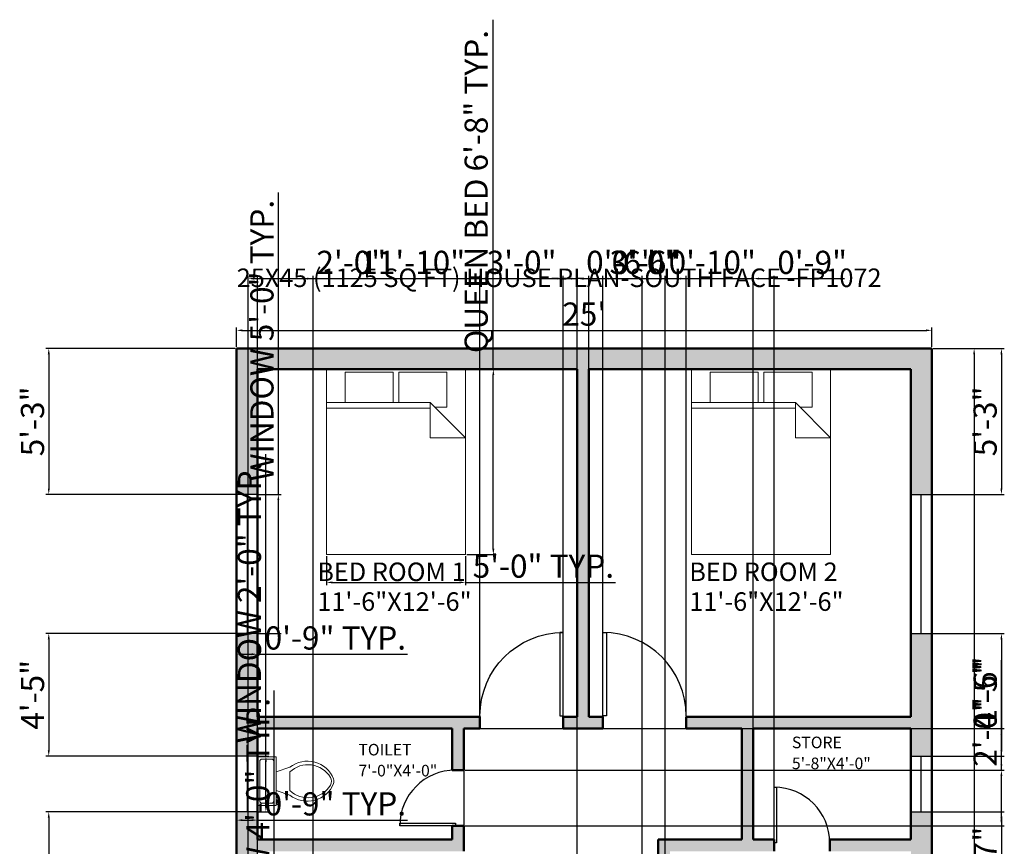
# Model space of a CAD drawing. Units: inches. Extents: x 3560 to 3985, y 1331 to 2044.
# Tile 2 of 2: x 3560 to 3985, y 1688 to 2044. Entities that reach past the tile are written whole.
import ezdxf

# ---------------------------------------------------------------- set-up
doc = ezdxf.new("R2010")
doc.units = ezdxf.units.IN
for name, color, linetype, lineweight in [('A-ANNO-DIMS', 5, 'Continuous', 18), ('A-ANNO-TEXT', 2, 'Continuous', 25), ('A-AREA-IDEN', 3, 'Continuous', 25), ('A-FLOR-FIXT', 9, 'Continuous', 18), ('A-FURN', 8, 'Continuous', 18), ('A-WALL-PATT', 7, 'Continuous', 13), ('DOOR', 6, 'Continuous', 25), ('WALL', 52, 'Continuous', 50), ('WINDOW', 4, 'Continuous', 25)]:
    doc.layers.add(name, color=color, linetype=linetype, lineweight=lineweight)
doc.styles.get("Standard").update_dxf_attribs({"font": 'arial.ttf'})
doc.dimstyles.new('ISO-25', dxfattribs={"dimtxt": 10, "dimasz": 2.5, "dimexe": 1.25, "dimexo": 0.625, "dimtad": 1, "dimdec": 1, "dimlunit": 3, "dimtxsty": 'Standard', "dimcen": 2.5, "dimadec": 0, "dimazin": 0, "dimtfac": 1, "dimtdec": 1, "dimtmove": 0, "dimatfit": 3, "dimfxl": 1, "dimarcsym": 0})

# ---------------------------------------------------------------- blocks, each defined once
blk = doc.blocks.new('*U5')
for p, q in [((0, 0), (0, -6)), ((40, 0), (40, -6))]:
    blk.add_line(p, q)
blk.add_lwpolyline([(0, 0), (0, 40), (1.75, 40), (1.75, 0)], close=True)
blk.add_arc((0, 0), 40, 0, 90)
blk = doc.blocks.new('*U7')
for p, q in [((9.5, -6), (9.5, -2)), ((-8, -8.5), (-8, -8)), ((-7, -8), (-7, -9.5)), ((-4, -8), (-6, -14)), ((4, -8), (6, -14)), ((-10, -8.5), (-8, -8.5)), ((-10, -9.5), (-10, -8.5)), ((-7, -9.5), (-10, -9.5)), ((4, -14), (-4, -14))]:
    blk.add_line(p, q)
blk.add_lwpolyline([(10.5, -8), (10.5, 0), (-10.5, 0), (-10.5, -8)], close=True)
for points in [[(-9.5, -2), (-9.5, -6)], [(8.5, -1), (-8.5, -1)], [(-8.5, -7), (8.5, -7)]]:
    blk.add_lwpolyline(points)
for centre, radius, start, end in [((-8.62, -1.88), 0.884, 81.8699, 188.1301), ((8.62, -1.88), 0.884, 351.8699, 98.1301), ((-8.62, -6.12), 0.884, 171.8699, 278.1301), ((8.62, -6.12), 0.884, 261.8699, 8.1301), ((3.52, -21.58), 12.17, 141.4691, 247.9714), ((4.2, -21.82), 11.33, 136.3677, 238.9468), ((-3.52, -21.58), 12.17, 292.0284, 38.5307), ((-4.2, -21.82), 11.33, 301.053, 43.6321), ((0, -27.88), 4, 245.7318, 294.2682), ((0, -29), 4, 254.8605, 285.1395)]:
    blk.add_arc(centre, radius, start, end)
blk = doc.blocks.new('Bed - Queen')
for p, q in [((0, -80.00003), (0, 0)), ((0, 0), (59.99999, 0)), ((59.99999, 0), (59.99999, -80.00003)), ((7.99999, -1.2), (28.79998, -1.2)), ((7.99999, -14.4), (7.99999, -1.2)), ((28.79998, -1.2), (28.79998, -14.4)), ((31.19999, -1.2), (51.99999, -1.2)), ((31.19999, -14.4), (31.19999, -1.2)), ((51.99999, -1.2), (51.99999, -16.4)), ((0, -14.4), (44.8, -14.4)), ((44.8, -16.8), (0, -16.8)), ((59.99999, -29.6), (44.8, -14.4)), ((44.8, -14.4), (44.8, -29.6)), ((51.99999, -16.4), (46.79936, -16.4)), ((44.8, -29.6), (59.99999, -29.6)), ((59.99999, -80.00003), (0, -80.00003))]:
    blk.add_line(p, q)
blk = doc.blocks.new('*D11')
at = {"layer": 'A-ANNO-DIMS', "color": 0, "lineweight": -2, "transparency": 16777216}
for p, q in [((3653.42, 1903.19), (3653.42, 1911.59)), ((3655.92, 1910.34), (3950.92, 1910.34)), ((3953.42, 1903.19), (3953.42, 1911.59))]:
    blk.add_line(p, q, dxfattribs=at)
at = {"layer": 'A-ANNO-DIMS', "color": 0, "transparency": 16777216}
for points in [[(3655.92, 1910.76), (3655.92, 1909.92), (3653.42, 1910.34)], [(3950.92, 1910.76), (3950.92, 1909.92), (3953.42, 1910.34)]]:
    blk.add_solid(points, dxfattribs=at)
at = {"layer": 'Defpoints', "color": 0, "transparency": 16777216}
for p in [(3953.42, 1910.34), (3653.42, 1902.56), (3953.42, 1902.56)]:
    blk.add_point(p, dxfattribs=at)
at = {"layer": 'A-ANNO-DIMS', "color": 0, "transparency": 16777216, "insert": (3803.42, 1916.07), "char_height": 10, "attachment_point": 5}
blk.add_mtext("25'", dxfattribs=at)
blk = doc.blocks.new('*D12')
at = {"layer": 'A-ANNO-DIMS', "color": 0, "lineweight": -2, "transparency": 16777216}
for p, q in [((3954.04, 1902.56), (3973, 1902.56)), ((3971.75, 1900.06), (3971.75, 1365.06)), ((3954.04, 1362.56), (3973, 1362.56))]:
    blk.add_line(p, q, dxfattribs=at)
at = {"layer": 'A-ANNO-DIMS', "color": 0, "transparency": 16777216}
for points in [[(3971.33, 1900.06), (3972.16, 1900.06), (3971.75, 1902.56)], [(3971.33, 1365.06), (3972.16, 1365.06), (3971.75, 1362.56)]]:
    blk.add_solid(points, dxfattribs=at)
at = {"layer": 'Defpoints', "color": 0, "transparency": 16777216}
for p in [(3953.42, 1902.56), (3953.42, 1362.56), (3971.75, 1362.56)]:
    blk.add_point(p, dxfattribs=at)
at = {"layer": 'A-ANNO-DIMS', "color": 0, "transparency": 16777216, "insert": (3966.04, 1633.18), "char_height": 10, "attachment_point": 5, "rotation": 90}
blk.add_mtext("45'", dxfattribs=at)
blk = doc.blocks.new('WIN-24IN')
for p, q in [((9, 24), (0, 24)), ((4.5, 24), (4.5, 0)), ((9, 0), (0, 0))]:
    blk.add_line(p, q)
blk = doc.blocks.new('WIN-60IN')
for p, q in [((9, 60), (0, 60)), ((4.5, 60), (4.5, 0)), ((9, 0), (0, 0))]:
    blk.add_line(p, q)
blk = doc.blocks.new('*D16')
at = {"layer": 'A-ANNO-DIMS', "color": 0, "lineweight": -2, "transparency": 16777216}
for p, q in [((3764.21, 1893.56), (3764.21, 2044.41)), ((3752.83, 1893.56), (3765.46, 1893.56)), ((3764.21, 1816.06), (3764.21, 1891.06)), ((3752.83, 1813.56), (3765.46, 1813.56))]:
    blk.add_line(p, q, dxfattribs=at)
at = {"layer": 'A-ANNO-DIMS', "color": 0, "transparency": 16777216}
for points in [[(3763.79, 1891.06), (3764.62, 1891.06), (3764.21, 1893.56)], [(3763.79, 1816.06), (3764.62, 1816.06), (3764.21, 1813.56)]]:
    blk.add_solid(points, dxfattribs=at)
at = {"layer": 'Defpoints', "color": 0, "transparency": 16777216}
for p in [(3752.21, 1893.56), (3764.21, 1893.56), (3752.21, 1813.56)]:
    blk.add_point(p, dxfattribs=at)
at = {"layer": 'A-ANNO-DIMS', "color": 0, "transparency": 16777216, "insert": (3758.1, 1970.24), "char_height": 10, "attachment_point": 5, "rotation": 90}
blk.add_mtext('QUEEN BED 6\'-8" TYP.', dxfattribs=at)
blk = doc.blocks.new('*D17')
at = {"layer": 'A-ANNO-DIMS', "color": 0, "lineweight": -2, "transparency": 16777216}
for p, q in [((3692.21, 1812.94), (3692.21, 1800.31)), ((3752.21, 1812.94), (3752.21, 1800.31)), ((3694.71, 1801.56), (3749.71, 1801.56)), ((3752.21, 1801.56), (3816.91, 1801.56))]:
    blk.add_line(p, q, dxfattribs=at)
at = {"layer": 'A-ANNO-DIMS', "color": 0, "transparency": 16777216}
for points in [[(3694.71, 1801.98), (3694.71, 1801.15), (3692.21, 1801.56)], [(3749.71, 1801.98), (3749.71, 1801.15), (3752.21, 1801.56)]]:
    blk.add_solid(points, dxfattribs=at)
at = {"layer": 'Defpoints', "color": 0, "transparency": 16777216}
for p in [(3692.21, 1813.56), (3752.21, 1813.56), (3752.21, 1801.56)]:
    blk.add_point(p, dxfattribs=at)
at = {"layer": 'A-ANNO-DIMS', "color": 0, "transparency": 16777216, "insert": (3785.81, 1807.29), "char_height": 10, "attachment_point": 5}
blk.add_mtext('5\'-0" TYP.', dxfattribs=at)
blk = doc.blocks.new('*D18')
at = {"layer": 'A-ANNO-DIMS', "color": 0, "lineweight": -2, "transparency": 16777216}
for p, q in [((3671.42, 1839.56), (3671.42, 1969.85)), ((3663.04, 1839.56), (3672.67, 1839.56)), ((3671.42, 1782.06), (3671.42, 1837.06)), ((3663.04, 1779.56), (3672.67, 1779.56))]:
    blk.add_line(p, q, dxfattribs=at)
at = {"layer": 'A-ANNO-DIMS', "color": 0, "transparency": 16777216}
for points in [[(3671, 1837.06), (3671.83, 1837.06), (3671.42, 1839.56)], [(3671, 1782.06), (3671.83, 1782.06), (3671.42, 1779.56)]]:
    blk.add_solid(points, dxfattribs=at)
at = {"layer": 'Defpoints', "color": 0, "transparency": 16777216}
for p in [(3662.42, 1839.56), (3671.42, 1839.56), (3662.42, 1779.56)]:
    blk.add_point(p, dxfattribs=at)
at = {"layer": 'A-ANNO-DIMS', "color": 0, "transparency": 16777216, "insert": (3665.62, 1905.96), "char_height": 10, "attachment_point": 5, "rotation": 90}
blk.add_mtext('WINDOW 5\'-0" TYP.', dxfattribs=at)
blk = doc.blocks.new('*D19')
at = {"layer": 'A-ANNO-DIMS', "color": 0, "lineweight": -2, "transparency": 16777216}
for p, q in [((3653.42, 1778.94), (3653.42, 1769.31)), ((3662.42, 1778.94), (3662.42, 1769.31)), ((3655.92, 1770.56), (3659.92, 1770.56)), ((3662.42, 1770.56), (3727.12, 1770.56))]:
    blk.add_line(p, q, dxfattribs=at)
at = {"layer": 'A-ANNO-DIMS', "color": 0, "transparency": 16777216}
for points in [[(3655.92, 1770.98), (3655.92, 1770.15), (3653.42, 1770.56)], [(3659.92, 1770.98), (3659.92, 1770.15), (3662.42, 1770.56)]]:
    blk.add_solid(points, dxfattribs=at)
at = {"layer": 'Defpoints', "color": 0, "transparency": 16777216}
for p in [(3653.42, 1779.56), (3662.42, 1779.56), (3662.42, 1770.56)]:
    blk.add_point(p, dxfattribs=at)
at = {"layer": 'A-ANNO-DIMS', "color": 0, "transparency": 16777216, "insert": (3696.02, 1776.29), "char_height": 10, "attachment_point": 5}
blk.add_mtext('0\'-9" TYP.', dxfattribs=at)
blk = doc.blocks.new('*D20')
at = {"layer": 'A-ANNO-DIMS', "color": 0, "lineweight": -2, "transparency": 16777216}
for p, q in [((3669.62, 1624.56), (3669.62, 1754.85)), ((3663.04, 1624.56), (3670.87, 1624.56)), ((3669.62, 1579.06), (3669.62, 1622.06)), ((3663.04, 1576.56), (3670.87, 1576.56))]:
    blk.add_line(p, q, dxfattribs=at)
at = {"layer": 'A-ANNO-DIMS', "color": 0, "transparency": 16777216}
for points in [[(3669.2, 1622.06), (3670.03, 1622.06), (3669.62, 1624.56)], [(3669.2, 1579.06), (3670.03, 1579.06), (3669.62, 1576.56)]]:
    blk.add_solid(points, dxfattribs=at)
at = {"layer": 'Defpoints', "color": 0, "transparency": 16777216}
for p in [(3662.42, 1624.56), (3669.62, 1624.56), (3662.42, 1576.56)]:
    blk.add_point(p, dxfattribs=at)
at = {"layer": 'A-ANNO-DIMS', "color": 0, "transparency": 16777216, "insert": (3663.82, 1690.96), "char_height": 10, "attachment_point": 5, "rotation": 90}
blk.add_mtext('WINDOW 4\'-0" TYP.', dxfattribs=at)
blk = doc.blocks.new('*D22')
at = {"layer": 'A-ANNO-DIMS', "color": 0, "lineweight": -2, "transparency": 16777216}
for p, q in [((3666.02, 1726.56), (3666.02, 1856.85)), ((3663.04, 1726.56), (3667.27, 1726.56)), ((3666.02, 1705.06), (3666.02, 1724.06)), ((3663.04, 1702.56), (3667.27, 1702.56))]:
    blk.add_line(p, q, dxfattribs=at)
at = {"layer": 'A-ANNO-DIMS', "color": 0, "transparency": 16777216}
for points in [[(3665.6, 1724.06), (3666.43, 1724.06), (3666.02, 1726.56)], [(3665.6, 1705.06), (3666.43, 1705.06), (3666.02, 1702.56)]]:
    blk.add_solid(points, dxfattribs=at)
at = {"layer": 'Defpoints', "color": 0, "transparency": 16777216}
for p in [(3662.42, 1726.56), (3666.02, 1726.56), (3662.42, 1702.56)]:
    blk.add_point(p, dxfattribs=at)
at = {"layer": 'A-ANNO-DIMS', "color": 0, "transparency": 16777216, "insert": (3660.22, 1792.96), "char_height": 10, "attachment_point": 5, "rotation": 90}
blk.add_mtext('WINDOW 2\'-0" TYP.', dxfattribs=at)
blk = doc.blocks.new('*D23')
at = {"layer": 'A-ANNO-DIMS', "color": 0, "lineweight": -2, "transparency": 16777216}
for p, q in [((3653.42, 1701.94), (3653.42, 1697.71)), ((3662.42, 1701.94), (3662.42, 1697.71)), ((3655.92, 1698.96), (3659.92, 1698.96)), ((3662.42, 1698.96), (3727.12, 1698.96))]:
    blk.add_line(p, q, dxfattribs=at)
at = {"layer": 'A-ANNO-DIMS', "color": 0, "transparency": 16777216}
for points in [[(3655.92, 1699.38), (3655.92, 1698.55), (3653.42, 1698.96)], [(3659.92, 1699.38), (3659.92, 1698.55), (3662.42, 1698.96)]]:
    blk.add_solid(points, dxfattribs=at)
at = {"layer": 'Defpoints', "color": 0, "transparency": 16777216}
for p in [(3653.42, 1702.56), (3662.42, 1702.56), (3662.42, 1698.96)]:
    blk.add_point(p, dxfattribs=at)
at = {"layer": 'A-ANNO-DIMS', "color": 0, "transparency": 16777216, "insert": (3696.02, 1704.69), "char_height": 10, "attachment_point": 5}
blk.add_mtext('0\'-9" TYP.', dxfattribs=at)
blk = doc.blocks.new('*D28')
at = {"layer": 'A-ANNO-DIMS', "color": 0, "lineweight": -2, "transparency": 16777216}
for p, q in [((3652.79, 1902.56), (3571.07, 1902.56)), ((3572.32, 1900.06), (3572.32, 1842.06)), ((3652.79, 1839.56), (3571.07, 1839.56))]:
    blk.add_line(p, q, dxfattribs=at)
at = {"layer": 'A-ANNO-DIMS', "color": 0, "transparency": 16777216}
for points in [[(3571.9, 1900.06), (3572.73, 1900.06), (3572.32, 1902.56)], [(3571.9, 1842.06), (3572.73, 1842.06), (3572.32, 1839.56)]]:
    blk.add_solid(points, dxfattribs=at)
at = {"layer": 'Defpoints', "color": 0, "transparency": 16777216}
for p in [(3653.42, 1902.56), (3572.32, 1839.56), (3653.42, 1839.56)]:
    blk.add_point(p, dxfattribs=at)
at = {"layer": 'A-ANNO-DIMS', "color": 0, "transparency": 16777216, "insert": (3566.58, 1871.06), "char_height": 10, "attachment_point": 5, "rotation": 90}
blk.add_mtext('5\'-3"', dxfattribs=at)
blk = doc.blocks.new('*D29')
at = {"layer": 'A-ANNO-DIMS', "color": 0, "lineweight": -2, "transparency": 16777216}
for p, q in [((3652.79, 1779.56), (3571.07, 1779.56)), ((3572.32, 1777.06), (3572.32, 1729.06)), ((3652.79, 1726.56), (3571.07, 1726.56))]:
    blk.add_line(p, q, dxfattribs=at)
at = {"layer": 'A-ANNO-DIMS', "color": 0, "transparency": 16777216}
for points in [[(3571.9, 1777.06), (3572.73, 1777.06), (3572.32, 1779.56)], [(3571.9, 1729.06), (3572.73, 1729.06), (3572.32, 1726.56)]]:
    blk.add_solid(points, dxfattribs=at)
at = {"layer": 'Defpoints', "color": 0, "transparency": 16777216}
for p in [(3653.42, 1779.56), (3572.32, 1726.56), (3653.42, 1726.56)]:
    blk.add_point(p, dxfattribs=at)
at = {"layer": 'A-ANNO-DIMS', "color": 0, "transparency": 16777216, "insert": (3566.61, 1753.06), "char_height": 10, "attachment_point": 5, "rotation": 90}
blk.add_mtext('4\'-5"', dxfattribs=at)
blk = doc.blocks.new('*D30')
at = {"layer": 'A-ANNO-DIMS', "color": 0, "lineweight": -2, "transparency": 16777216}
for p, q in [((3652.79, 1702.56), (3571.07, 1702.56)), ((3572.32, 1700.06), (3572.32, 1627.06)), ((3652.79, 1624.56), (3571.07, 1624.56))]:
    blk.add_line(p, q, dxfattribs=at)
at = {"layer": 'A-ANNO-DIMS', "color": 0, "transparency": 16777216}
for points in [[(3571.9, 1700.06), (3572.73, 1700.06), (3572.32, 1702.56)], [(3571.9, 1627.06), (3572.73, 1627.06), (3572.32, 1624.56)]]:
    blk.add_solid(points, dxfattribs=at)
at = {"layer": 'Defpoints', "color": 0, "transparency": 16777216}
for p in [(3653.42, 1702.56), (3572.32, 1624.56), (3653.42, 1624.56)]:
    blk.add_point(p, dxfattribs=at)
at = {"layer": 'A-ANNO-DIMS', "color": 0, "transparency": 16777216, "insert": (3566.59, 1663.56), "char_height": 10, "attachment_point": 5, "rotation": 90}
blk.add_mtext('6\'-6"', dxfattribs=at)
blk = doc.blocks.new('*D31')
at = {"layer": 'A-ANNO-DIMS', "color": 0, "lineweight": -2, "transparency": 16777216}
for p, q in [((3954.04, 1902.56), (3984.77, 1902.56)), ((3983.52, 1900.06), (3983.52, 1842.06)), ((3954.04, 1839.56), (3984.77, 1839.56))]:
    blk.add_line(p, q, dxfattribs=at)
at = {"layer": 'A-ANNO-DIMS', "color": 0, "transparency": 16777216}
for points in [[(3983.1, 1900.06), (3983.93, 1900.06), (3983.52, 1902.56)], [(3983.1, 1842.06), (3983.93, 1842.06), (3983.52, 1839.56)]]:
    blk.add_solid(points, dxfattribs=at)
at = {"layer": 'Defpoints', "color": 0, "transparency": 16777216}
for p in [(3953.42, 1902.56), (3953.42, 1839.56), (3983.52, 1839.56)]:
    blk.add_point(p, dxfattribs=at)
at = {"layer": 'A-ANNO-DIMS', "color": 0, "transparency": 16777216, "insert": (3977.78, 1871.06), "char_height": 10, "attachment_point": 5, "rotation": 90}
blk.add_mtext('5\'-3"', dxfattribs=at)
blk = doc.blocks.new('*D32')
at = {"layer": 'A-ANNO-DIMS', "color": 0, "lineweight": -2, "transparency": 16777216}
for p, q in [((3954.04, 1779.56), (3984.77, 1779.56)), ((3983.52, 1777.06), (3983.52, 1729.06)), ((3954.04, 1726.56), (3984.77, 1726.56))]:
    blk.add_line(p, q, dxfattribs=at)
at = {"layer": 'A-ANNO-DIMS', "color": 0, "transparency": 16777216}
for points in [[(3983.1, 1777.06), (3983.93, 1777.06), (3983.52, 1779.56)], [(3983.1, 1729.06), (3983.93, 1729.06), (3983.52, 1726.56)]]:
    blk.add_solid(points, dxfattribs=at)
at = {"layer": 'Defpoints', "color": 0, "transparency": 16777216}
for p in [(3953.42, 1779.56), (3953.42, 1726.56), (3983.52, 1726.56)]:
    blk.add_point(p, dxfattribs=at)
at = {"layer": 'A-ANNO-DIMS', "color": 0, "transparency": 16777216, "insert": (3977.81, 1753.06), "char_height": 10, "attachment_point": 5, "rotation": 90}
blk.add_mtext('4\'-5"', dxfattribs=at)
blk = doc.blocks.new('*D33')
at = {"layer": 'A-ANNO-DIMS', "color": 0, "lineweight": -2, "transparency": 16777216}
for p, q in [((3954.04, 1702.56), (3984.77, 1702.56)), ((3983.52, 1700.06), (3983.52, 1662.06)), ((3954.04, 1659.56), (3984.77, 1659.56))]:
    blk.add_line(p, q, dxfattribs=at)
at = {"layer": 'A-ANNO-DIMS', "color": 0, "transparency": 16777216}
for points in [[(3983.1, 1700.06), (3983.93, 1700.06), (3983.52, 1702.56)], [(3983.1, 1662.06), (3983.93, 1662.06), (3983.52, 1659.56)]]:
    blk.add_solid(points, dxfattribs=at)
at = {"layer": 'Defpoints', "color": 0, "transparency": 16777216}
for p in [(3953.42, 1702.56), (3953.42, 1659.56), (3983.52, 1659.56)]:
    blk.add_point(p, dxfattribs=at)
at = {"layer": 'A-ANNO-DIMS', "color": 0, "transparency": 16777216, "insert": (3977.78, 1681.06), "char_height": 10, "attachment_point": 5, "rotation": 90}
blk.add_mtext('3\'-7"', dxfattribs=at)
blk = doc.blocks.new('*D36')
at = {"layer": 'A-ANNO-DIMS', "color": 0, "lineweight": -2, "transparency": 16777216}
for p, q in [((3662.42, 1517.19), (3662.42, 1933.91)), ((3686.42, 1517.19), (3686.42, 1933.91)), ((3664.92, 1932.66), (3683.92, 1932.66)), ((3686.42, 1932.66), (3716.92, 1932.66))]:
    blk.add_line(p, q, dxfattribs=at)
at = {"layer": 'A-ANNO-DIMS', "color": 0, "transparency": 16777216}
for points in [[(3664.92, 1933.08), (3664.92, 1932.25), (3662.42, 1932.66)], [(3683.92, 1933.08), (3683.92, 1932.25), (3686.42, 1932.66)]]:
    blk.add_solid(points, dxfattribs=at)
at = {"layer": 'Defpoints', "color": 0, "transparency": 16777216}
for p in [(3686.42, 1932.66), (3662.42, 1516.56), (3686.42, 1516.56)]:
    blk.add_point(p, dxfattribs=at)
at = {"layer": 'A-ANNO-DIMS', "color": 0, "transparency": 16777216, "insert": (3702.92, 1938.39), "char_height": 10, "attachment_point": 5}
blk.add_mtext('2\'-0"', dxfattribs=at)
blk = doc.blocks.new('*D40')
at = {"layer": 'A-ANNO-DIMS', "color": 0, "lineweight": -2, "transparency": 16777216}
for p, q in [((3758.42, 1744.19), (3758.42, 1933.91)), ((3794.42, 1744.19), (3794.42, 1933.91)), ((3760.92, 1932.66), (3791.92, 1932.66))]:
    blk.add_line(p, q, dxfattribs=at)
at = {"layer": 'A-ANNO-DIMS', "color": 0, "transparency": 16777216}
for points in [[(3760.92, 1933.08), (3760.92, 1932.25), (3758.42, 1932.66)], [(3791.92, 1933.08), (3791.92, 1932.25), (3794.42, 1932.66)]]:
    blk.add_solid(points, dxfattribs=at)
at = {"layer": 'Defpoints', "color": 0, "transparency": 16777216}
for p in [(3794.42, 1932.66), (3758.42, 1743.56), (3794.42, 1743.56)]:
    blk.add_point(p, dxfattribs=at)
at = {"layer": 'A-ANNO-DIMS', "color": 0, "transparency": 16777216, "insert": (3776.42, 1938.4), "char_height": 10, "attachment_point": 5}
blk.add_mtext('3\'-0"', dxfattribs=at)
blk = doc.blocks.new('*D41')
at = {"layer": 'A-ANNO-DIMS', "color": 0, "lineweight": -2, "transparency": 16777216}
for p, q in [((3794.42, 1744.19), (3794.42, 1933.91)), ((3800.42, 1744.19), (3800.42, 1933.91)), ((3791.92, 1932.66), (3789.42, 1932.66)), ((3794.42, 1932.66), (3800.42, 1932.66)), ((3802.92, 1932.66), (3833.25, 1932.66))]:
    blk.add_line(p, q, dxfattribs=at)
at = {"layer": 'A-ANNO-DIMS', "color": 0, "transparency": 16777216}
for points in [[(3791.92, 1933.08), (3791.92, 1932.25), (3794.42, 1932.66)], [(3802.92, 1933.08), (3802.92, 1932.25), (3800.42, 1932.66)]]:
    blk.add_solid(points, dxfattribs=at)
at = {"layer": 'Defpoints', "color": 0, "transparency": 16777216}
for p in [(3800.42, 1932.66), (3794.42, 1743.56), (3800.42, 1743.56)]:
    blk.add_point(p, dxfattribs=at)
at = {"layer": 'A-ANNO-DIMS', "color": 0, "transparency": 16777216, "insert": (3819.33, 1938.39), "char_height": 10, "attachment_point": 5}
blk.add_mtext('0\'-6"', dxfattribs=at)
blk = doc.blocks.new('*D42')
at = {"layer": 'A-ANNO-DIMS', "color": 0, "lineweight": -2, "transparency": 16777216}
for p, q in [((3805.42, 1744.19), (3805.42, 1933.91)), ((3811.42, 1744.19), (3811.42, 1933.91)), ((3802.92, 1932.66), (3800.42, 1932.66)), ((3805.42, 1932.66), (3811.42, 1932.66)), ((3813.92, 1932.66), (3844.25, 1932.66))]:
    blk.add_line(p, q, dxfattribs=at)
at = {"layer": 'A-ANNO-DIMS', "color": 0, "transparency": 16777216}
for points in [[(3802.92, 1933.08), (3802.92, 1932.25), (3805.42, 1932.66)], [(3813.92, 1933.08), (3813.92, 1932.25), (3811.42, 1932.66)]]:
    blk.add_solid(points, dxfattribs=at)
at = {"layer": 'Defpoints', "color": 0, "transparency": 16777216}
for p in [(3811.42, 1932.66), (3805.42, 1743.56), (3811.42, 1743.56)]:
    blk.add_point(p, dxfattribs=at)
at = {"layer": 'A-ANNO-DIMS', "color": 0, "transparency": 16777216, "insert": (3830.33, 1938.39), "char_height": 10, "attachment_point": 5}
blk.add_mtext('0\'-6"', dxfattribs=at)
blk = doc.blocks.new('*D43')
at = {"layer": 'A-ANNO-DIMS', "color": 0, "lineweight": -2, "transparency": 16777216}
for p, q in [((3811.42, 1744.19), (3811.42, 1933.91)), ((3847.42, 1744.19), (3847.42, 1933.91)), ((3813.92, 1932.66), (3844.92, 1932.66))]:
    blk.add_line(p, q, dxfattribs=at)
at = {"layer": 'A-ANNO-DIMS', "color": 0, "transparency": 16777216}
for points in [[(3813.92, 1933.08), (3813.92, 1932.25), (3811.42, 1932.66)], [(3844.92, 1933.08), (3844.92, 1932.25), (3847.42, 1932.66)]]:
    blk.add_solid(points, dxfattribs=at)
at = {"layer": 'Defpoints', "color": 0, "transparency": 16777216}
for p in [(3847.42, 1932.66), (3811.42, 1743.56), (3847.42, 1743.56)]:
    blk.add_point(p, dxfattribs=at)
at = {"layer": 'A-ANNO-DIMS', "color": 0, "transparency": 16777216, "insert": (3829.42, 1938.4), "char_height": 10, "attachment_point": 5}
blk.add_mtext('3\'-0"', dxfattribs=at)
blk = doc.blocks.new('*D45')
at = {"layer": 'A-ANNO-DIMS', "color": 0, "lineweight": -2, "transparency": 16777216}
for p, q in [((3876.42, 1691.19), (3876.42, 1933.91)), ((3885.42, 1691.19), (3885.42, 1933.91)), ((3878.92, 1932.66), (3882.92, 1932.66)), ((3885.42, 1932.66), (3915.75, 1932.66))]:
    blk.add_line(p, q, dxfattribs=at)
at = {"layer": 'A-ANNO-DIMS', "color": 0, "transparency": 16777216}
for points in [[(3878.92, 1933.08), (3878.92, 1932.25), (3876.42, 1932.66)], [(3882.92, 1933.08), (3882.92, 1932.25), (3885.42, 1932.66)]]:
    blk.add_solid(points, dxfattribs=at)
at = {"layer": 'Defpoints', "color": 0, "transparency": 16777216}
for p in [(3885.42, 1932.66), (3876.42, 1690.56), (3885.42, 1690.56)]:
    blk.add_point(p, dxfattribs=at)
at = {"layer": 'A-ANNO-DIMS', "color": 0, "transparency": 16777216, "insert": (3901.83, 1938.39), "char_height": 10, "attachment_point": 5}
blk.add_mtext('0\'-9"', dxfattribs=at)
blk = doc.blocks.new('*D47')
at = {"layer": 'A-ANNO-DIMS', "color": 0, "lineweight": -2, "transparency": 16777216}
for p, q in [((3983.52, 1720.56), (3983.52, 1751.07)), ((3752.04, 1720.56), (3984.77, 1720.56)), ((3983.52, 1699.06), (3983.52, 1718.06)), ((3752.04, 1696.56), (3984.77, 1696.56))]:
    blk.add_line(p, q, dxfattribs=at)
at = {"layer": 'A-ANNO-DIMS', "color": 0, "transparency": 16777216}
for points in [[(3983.1, 1718.06), (3983.93, 1718.06), (3983.52, 1720.56)], [(3983.1, 1699.06), (3983.93, 1699.06), (3983.52, 1696.56)]]:
    blk.add_solid(points, dxfattribs=at)
at = {"layer": 'Defpoints', "color": 0, "transparency": 16777216}
for p in [(3751.42, 1720.56), (3983.52, 1720.56), (3751.42, 1696.56)]:
    blk.add_point(p, dxfattribs=at)
at = {"layer": 'A-ANNO-DIMS', "color": 0, "transparency": 16777216, "insert": (3977.79, 1737.06), "char_height": 10, "attachment_point": 5, "rotation": 90}
blk.add_mtext('2\'-0"', dxfattribs=at)
blk = doc.blocks.new('*D48')
at = {"layer": 'A-ANNO-DIMS', "color": 0, "lineweight": -2, "transparency": 16777216}
for p, q in [((3983.52, 1738.56), (3983.52, 1767.95)), ((3752.04, 1738.56), (3984.77, 1738.56)), ((3983.52, 1723.06), (3983.52, 1736.06)), ((3752.04, 1720.56), (3984.77, 1720.56))]:
    blk.add_line(p, q, dxfattribs=at)
at = {"layer": 'A-ANNO-DIMS', "color": 0, "transparency": 16777216}
for points in [[(3983.1, 1736.06), (3983.93, 1736.06), (3983.52, 1738.56)], [(3983.1, 1723.06), (3983.93, 1723.06), (3983.52, 1720.56)]]:
    blk.add_solid(points, dxfattribs=at)
at = {"layer": 'Defpoints', "color": 0, "transparency": 16777216}
for p in [(3751.42, 1738.56), (3983.52, 1738.56), (3751.42, 1720.56)]:
    blk.add_point(p, dxfattribs=at)
at = {"layer": 'A-ANNO-DIMS', "color": 0, "transparency": 16777216, "insert": (3977.79, 1754.51), "char_height": 10, "attachment_point": 5, "rotation": 90}
blk.add_mtext('1\'-6"', dxfattribs=at)
blk = doc.blocks.new('*D52')
at = {"layer": 'A-ANNO-DIMS', "color": 0, "lineweight": -2, "transparency": 16777216}
for p, q in [((3658.42, 1372.19), (3658.42, 1933.91)), ((3800.42, 1372.19), (3800.42, 1933.91)), ((3660.92, 1932.66), (3797.92, 1932.66))]:
    blk.add_line(p, q, dxfattribs=at)
at = {"layer": 'A-ANNO-DIMS', "color": 0, "transparency": 16777216}
for points in [[(3660.92, 1933.08), (3660.92, 1932.25), (3658.42, 1932.66)], [(3797.92, 1933.08), (3797.92, 1932.25), (3800.42, 1932.66)]]:
    blk.add_solid(points, dxfattribs=at)
at = {"layer": 'Defpoints', "color": 0, "transparency": 16777216}
for p in [(3800.42, 1932.66), (3658.42, 1371.56), (3800.42, 1371.56)]:
    blk.add_point(p, dxfattribs=at)
at = {"layer": 'A-ANNO-DIMS', "color": 0, "transparency": 16777216, "insert": (3729.42, 1938.39), "char_height": 10, "attachment_point": 5}
blk.add_mtext('11\'-10"', dxfattribs=at)
blk = doc.blocks.new('*D53')
at = {"layer": 'A-ANNO-DIMS', "color": 0, "lineweight": -2, "transparency": 16777216}
for p, q in [((3828.42, 1372.19), (3828.42, 1933.91)), ((3838.42, 1372.19), (3838.42, 1933.91)), ((3830.92, 1932.66), (3835.92, 1932.66)), ((3838.42, 1932.66), (3876.52, 1932.66))]:
    blk.add_line(p, q, dxfattribs=at)
at = {"layer": 'A-ANNO-DIMS', "color": 0, "transparency": 16777216}
for points in [[(3830.92, 1933.08), (3830.92, 1932.25), (3828.42, 1932.66)], [(3835.92, 1933.08), (3835.92, 1932.25), (3838.42, 1932.66)]]:
    blk.add_solid(points, dxfattribs=at)
at = {"layer": 'Defpoints', "color": 0, "transparency": 16777216}
for p in [(3838.42, 1932.66), (3828.42, 1371.56), (3838.42, 1371.56)]:
    blk.add_point(p, dxfattribs=at)
at = {"layer": 'A-ANNO-DIMS', "color": 0, "transparency": 16777216, "insert": (3858.72, 1938.39), "char_height": 10, "attachment_point": 5}
blk.add_mtext('0\'-10"', dxfattribs=at)

msp = doc.modelspace()

# ---------------------------------------------------------------- hatches: boundary and pattern name
at = {"layer": 'A-WALL-PATT'}
h = msp.add_hatch(color=256, dxfattribs=at)
h.dxf.hatch_style = 1
h.paths.add_polyline_path([(3953.42, 1902.56), (3653.42, 1902.56), (3653.42, 1839.56), (3662.42, 1839.56), (3662.42, 1893.56), (3800.42, 1893.56), (3800.42, 1743.56), (3794.42, 1743.56), (3794.42, 1738.56), (3800.42, 1738.56), (3811.42, 1738.56), (3811.42, 1743.56), (3805.42, 1743.56), (3805.42, 1893.56), (3944.42, 1893.56), (3944.42, 1839.56), (3953.42, 1839.56)])
h = msp.add_hatch(color=256, dxfattribs=at)
h.dxf.hatch_style = 1
h.paths.add_polyline_path([(3758.42, 1743.56), (3662.42, 1743.56), (3662.42, 1779.56), (3653.42, 1779.56), (3653.42, 1726.56), (3662.42, 1726.56), (3662.42, 1738.56), (3746.42, 1738.56), (3746.42, 1720.56), (3751.42, 1720.56), (3751.42, 1738.56), (3758.42, 1738.56)])
h = msp.add_hatch(color=256, dxfattribs=at)
h.dxf.hatch_style = 1
h.paths.add_polyline_path([(3953.42, 1779.56), (3944.42, 1779.56), (3944.42, 1743.56), (3847.42, 1743.56), (3847.42, 1738.56), (3871.42, 1738.56), (3871.42, 1690.56), (3835.42, 1690.56), (3835.42, 1679.56), (3840.42, 1679.56), (3840.42, 1685.56), (3885.42, 1685.56), (3885.42, 1689.16), (3885.42, 1690.56), (3876.42, 1690.56), (3876.42, 1738.56), (3944.42, 1738.56), (3944.42, 1726.56), (3953.42, 1726.56)])
h = msp.add_hatch(color=256, dxfattribs=at)
h.dxf.hatch_style = 1
h.paths.add_polyline_path([(3662.42, 1685.56), (3751.42, 1685.56), (3751.42, 1696.56), (3747.82, 1696.56), (3746.42, 1696.56), (3746.42, 1690.56), (3662.42, 1690.56), (3662.42, 1702.56), (3653.42, 1702.56), (3653.42, 1624.56), (3662.42, 1624.56)])
h = msp.add_hatch(color=256, dxfattribs=at)
h.dxf.hatch_style = 1
h.paths.add_polyline_path([(3953.42, 1702.56), (3944.42, 1702.56), (3944.42, 1690.56), (3909.42, 1690.56), (3909.42, 1685.56), (3944.42, 1685.56), (3944.42, 1659.56), (3953.42, 1659.56)])

# ---------------------------------------------------------------- linework, layer by layer
at = {"layer": 'DOOR'}
for p, q in [((3758.42, 1738.56), (3794.42, 1738.56)), ((3811.42, 1738.56), (3847.42, 1738.56)), ((3751.42, 1720.56), (3751.42, 1696.56))]:
    msp.add_line(p, q, dxfattribs=at)
at = {"layer": 'WALL'}
for p, q in [((3653.42, 1902.56), (3953.42, 1902.56)), ((3653.42, 1902.56), (3653.42, 1362.56)), ((3953.42, 1902.56), (3953.42, 1362.56)), ((3662.42, 1893.56), (3800.42, 1893.56)), ((3662.42, 1893.56), (3662.42, 1743.56)), ((3800.42, 1893.56), (3800.42, 1743.56)), ((3805.42, 1893.56), (3805.42, 1743.56)), ((3805.42, 1893.56), (3944.42, 1893.56)), ((3944.42, 1893.56), (3944.42, 1743.56)), ((3662.42, 1743.56), (3758.42, 1743.56)), ((3758.42, 1743.56), (3758.42, 1738.56)), ((3794.42, 1743.56), (3794.42, 1738.56)), ((3794.42, 1743.56), (3800.42, 1743.56)), ((3805.42, 1743.56), (3811.42, 1743.56)), ((3811.42, 1743.56), (3811.42, 1738.56)), ((3847.42, 1743.56), (3847.42, 1738.56)), ((3847.42, 1743.56), (3944.42, 1743.56)), ((3662.42, 1738.56), (3746.42, 1738.56)), ((3662.42, 1738.56), (3662.42, 1690.56)), ((3746.42, 1738.56), (3746.42, 1720.56)), ((3751.42, 1738.56), (3751.42, 1720.56)), ((3751.42, 1738.56), (3758.42, 1738.56)), ((3794.42, 1738.56), (3800.42, 1738.56)), ((3800.42, 1738.56), (3811.42, 1738.56)), ((3847.42, 1738.56), (3871.42, 1738.56)), ((3871.42, 1738.56), (3871.42, 1690.56)), ((3876.42, 1738.56), (3876.42, 1690.56)), ((3876.42, 1738.56), (3944.42, 1738.56)), ((3944.42, 1738.56), (3944.42, 1690.56)), ((3746.42, 1720.56), (3751.42, 1720.56)), ((3746.42, 1696.56), (3751.42, 1696.56)), ((3746.42, 1696.56), (3746.42, 1690.56)), ((3751.42, 1696.56), (3751.42, 1685.56)), ((3662.42, 1690.56), (3746.42, 1690.56)), ((3835.42, 1690.56), (3871.42, 1690.56)), ((3835.42, 1690.56), (3835.42, 1679.56)), ((3876.42, 1690.56), (3885.42, 1690.56)), ((3885.42, 1690.56), (3885.42, 1685.56)), ((3909.42, 1690.56), (3909.42, 1685.56)), ((3909.42, 1690.56), (3944.42, 1690.56))]:
    msp.add_line(p, q, dxfattribs=at)

# ---------------------------------------------------------------- block references
at = {"layer": 'A-FLOR-FIXT', "rotation": 90}
msp.add_blockref('*U7', (3662.42, 1715.76), dxfattribs=at)
at = {"layer": 'A-FURN'}
for p in [(3692.21, 1893.56), (3849.77, 1893.56)]:
    msp.add_blockref('Bed - Queen', p, dxfattribs=at)
at = {"layer": 'DOOR'}
for p, xscale, yscale, zscale in [((3794.42, 1743.96), -0.8999999999999898, 0.8999999999999898, 0.8999999999999898), ((3811.42, 1743.96), 0.8999999999999898, 0.8999999999999898, 0.8999999999999898), ((3885.42, 1689.16), 0.5999999999999819, 0.5999999999999819, 0.5999999999999819)]:
    msp.add_blockref('*U5', p, dxfattribs=dict(at, xscale=xscale, yscale=yscale, zscale=zscale))
at = {"layer": 'DOOR', "xscale": 0.5999999999999782, "yscale": 0.5999999999999782, "zscale": 0.5999999999999782, "rotation": 89.99999999999902}
msp.add_blockref('*U5', (3747.82, 1696.56), dxfattribs=at)
at = {"layer": 'WINDOW'}
for name, p in [('WIN-60IN', (3653.42, 1779.56)), ('WIN-24IN', (3653.42, 1702.56))]:
    msp.add_blockref(name, p, dxfattribs=at)
at = {"layer": 'WINDOW', "rotation": 180}
for name, p in [('WIN-60IN', (3953.42, 1839.56)), ('WIN-24IN', (3953.42, 1726.56))]:
    msp.add_blockref(name, p, dxfattribs=at)

# ---------------------------------------------------------------- texts
at = {"layer": 'A-ANNO-TEXT'}
msp.add_text('25X45 (1125 SQ FT) HOUSE PLAN-SOUTH FACE -FP1072', height=8, dxfattribs=at).set_placement((3653.45, 1929.03))
at = {"layer": 'A-AREA-IDEN'}
for s, height, p in [('BED ROOM 1', 8, (3688.23, 1802.14)), ('BED ROOM 2', 8, (3848.79, 1802.14)), ('11\'-6"X12\'-6"', 8, (3688.23, 1789.29)), ('11\'-6"X12\'-6"', 8, (3848.79, 1789.29)), ('STORE', 5, (3893.09, 1730)), ('TOILET', 5, (3705.97, 1726.88)), ('5\'-8"X4\'-0"', 5, (3893.09, 1720.96)), ('7\'-0"X4\'-0"', 5, (3705.97, 1717.84))]:
    msp.add_text(s, height=height, dxfattribs=at).set_placement(p)

# ---------------------------------------------------------------- dimensions: what is measured, and where the dimension line sits
at = {"layer": 'A-ANNO-DIMS'}
for base, p1, p2, text, picture, middle in [((3764.21, 1893.56), (3752.21, 1813.56), (3752.21, 1893.56), 'QUEEN BED <> TYP.', '*D16', (3758.1, 1970.24)), ((3671.42, 1839.56), (3662.42, 1779.56), (3662.42, 1839.56), 'WINDOW <> TYP.', '*D18', (3665.62, 1905.96)), ((3666.02, 1726.56), (3662.42, 1702.56), (3662.42, 1726.56), 'WINDOW <> TYP.', '*D22', (3660.22, 1792.96)), ((3669.62, 1624.56), (3662.42, 1576.56), (3662.42, 1624.56), 'WINDOW <> TYP.', '*D20', (3663.82, 1690.96))]:
    dim = msp.add_linear_dim(base=base, p1=p1, p2=p2, angle=90, text=text, dimstyle='ISO-25', override={"dimdec": 1, "dimlfac": 1, "dimrnd": 0, "dimzin": 1, "dimdsep": 46, "dimlunit": 4, "dimfrac": 2}, dxfattribs=at)
    dim.commit()
    dim.dimension.update_dxf_attribs({"geometry": picture, "text_midpoint": middle})
for base, p1, p2, override, picture, middle in [((3800.42, 1932.66), (3658.42, 1371.56), (3800.42, 1371.56), {"dimdec": 1, "dimlfac": 1, "dimrnd": 0, "dimzin": 1, "dimdsep": 46, "dimlunit": 4, "dimfrac": 2}, '*D52', (3729.42, 1938.39)), ((3686.42, 1932.66), (3662.42, 1516.56), (3686.42, 1516.56), {"dimdec": 1, "dimlfac": 1, "dimrnd": 0, "dimzin": 1, "dimdsep": 46, "dimlunit": 4, "dimfrac": 2}, '*D36', (3702.92, 1938.39)), ((3794.42, 1932.66), (3758.42, 1743.56), (3794.42, 1743.56), {"dimdec": 1, "dimlfac": 1, "dimrnd": 0, "dimzin": 1, "dimdsep": 46, "dimlunit": 4, "dimfrac": 2}, '*D40', (3776.42, 1938.4)), ((3800.42, 1932.66), (3794.42, 1743.56), (3800.42, 1743.56), {"dimdec": 1, "dimlfac": 1, "dimrnd": 0, "dimzin": 1, "dimdsep": 46, "dimlunit": 4, "dimfrac": 2}, '*D41', (3819.33, 1938.39)), ((3811.42, 1932.66), (3805.42, 1743.56), (3811.42, 1743.56), {"dimdec": 1, "dimlfac": 1, "dimrnd": 0, "dimzin": 1, "dimdsep": 46, "dimlunit": 4, "dimfrac": 2}, '*D42', (3830.33, 1938.39)), ((3847.42, 1932.66), (3811.42, 1743.56), (3847.42, 1743.56), {"dimdec": 1, "dimlfac": 1, "dimrnd": 0, "dimzin": 1, "dimdsep": 46, "dimlunit": 4, "dimfrac": 2}, '*D43', (3829.42, 1938.4)), ((3838.42, 1932.66), (3828.42, 1371.56), (3838.42, 1371.56), {"dimdec": 1, "dimlfac": 1, "dimrnd": 0, "dimzin": 1, "dimdsep": 46, "dimlunit": 4, "dimfrac": 2}, '*D53', (3858.72, 1938.39)), ((3885.42, 1932.66), (3876.42, 1690.56), (3885.42, 1690.56), {"dimdec": 1, "dimlfac": 1, "dimrnd": 0, "dimzin": 1, "dimdsep": 46, "dimlunit": 4, "dimfrac": 2}, '*D45', (3901.83, 1938.39)), ((3953.42, 1910.34), (3653.42, 1902.56), (3953.42, 1902.56), {"dimclrd": 0, "dimclre": 0, "dimclrt": 0}, '*D11', (3803.42, 1916.07))]:
    dim = msp.add_linear_dim(base=base, p1=p1, p2=p2, dimstyle='ISO-25', override=override, dxfattribs=at)
    dim.commit()
    dim.dimension.update_dxf_attribs({"geometry": picture, "text_midpoint": middle})
for base, p1, p2, picture, middle in [((3572.32, 1839.56), (3653.42, 1902.56), (3653.42, 1839.56), '*D28', (3566.58, 1871.06)), ((3983.52, 1839.56), (3953.42, 1902.56), (3953.42, 1839.56), '*D31', (3977.78, 1871.06)), ((3572.32, 1726.56), (3653.42, 1779.56), (3653.42, 1726.56), '*D29', (3566.61, 1753.06)), ((3983.52, 1726.56), (3953.42, 1779.56), (3953.42, 1726.56), '*D32', (3977.81, 1753.06)), ((3983.52, 1738.56), (3751.42, 1720.56), (3751.42, 1738.56), '*D48', (3977.79, 1754.51)), ((3983.52, 1720.56), (3751.42, 1696.56), (3751.42, 1720.56), '*D47', (3977.79, 1737.06)), ((3572.32, 1624.56), (3653.42, 1702.56), (3653.42, 1624.56), '*D30', (3566.59, 1663.56)), ((3983.52, 1659.56), (3953.42, 1702.56), (3953.42, 1659.56), '*D33', (3977.78, 1681.06))]:
    dim = msp.add_linear_dim(base=base, p1=p1, p2=p2, angle=90, dimstyle='ISO-25', override={"dimdec": 1, "dimlfac": 1, "dimrnd": 0, "dimzin": 1, "dimdsep": 46, "dimlunit": 4, "dimfrac": 2}, dxfattribs=at)
    dim.commit()
    dim.dimension.update_dxf_attribs({"geometry": picture, "text_midpoint": middle})
dim = msp.add_linear_dim(base=(3971.75, 1362.56), p1=(3953.42, 1902.56), p2=(3953.42, 1362.56), angle=90, dimstyle='ISO-25', override={"dimclrd": 0, "dimclre": 0, "dimclrt": 0}, dxfattribs=at)
dim.commit()
dim.dimension.update_dxf_attribs({"geometry": '*D12', "text_midpoint": (3971.75, 1633.18), "dimtype": 160})
for base, p1, p2, picture, middle in [((3752.21, 1801.56), (3692.21, 1813.56), (3752.21, 1813.56), '*D17', (3785.81, 1807.29)), ((3662.42, 1770.56), (3653.42, 1779.56), (3662.42, 1779.56), '*D19', (3696.02, 1776.29)), ((3662.42, 1698.96), (3653.42, 1702.56), (3662.42, 1702.56), '*D23', (3696.02, 1704.69))]:
    dim = msp.add_linear_dim(base=base, p1=p1, p2=p2, text='<> TYP.', dimstyle='ISO-25', override={"dimdec": 1, "dimlfac": 1, "dimrnd": 0, "dimzin": 1, "dimdsep": 46, "dimlunit": 4, "dimfrac": 2}, dxfattribs=at)
    dim.commit()
    dim.dimension.update_dxf_attribs({"geometry": picture, "text_midpoint": middle})

doc.saveas('drawing.dxf')
